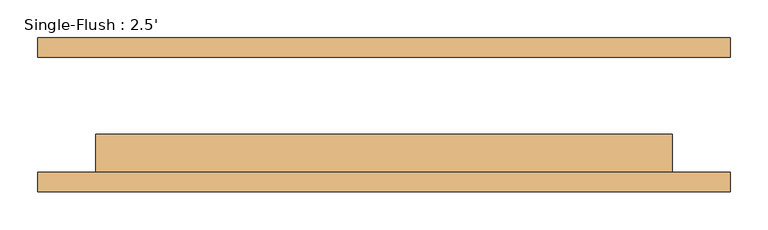
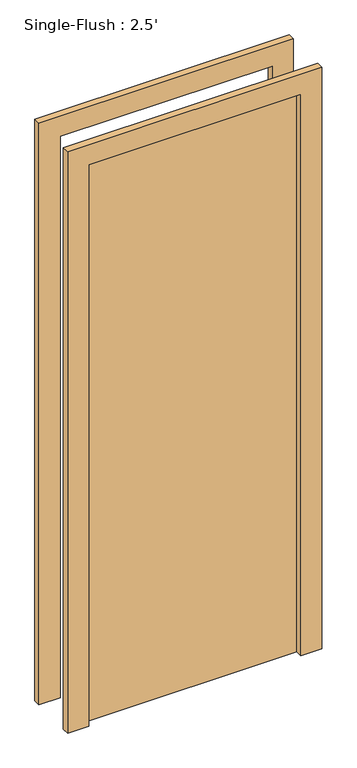
"""IFC4 building model written with IfcOpenShell, lengths in millimetres: door geometry, Single-Flush : 2.5'."""

from ifc_helpers import new_model, si_unit, frame, origin, origin_with_axes, place, context, project, spatial, polyline, outline, extrude, source, transform, mapped, element, save


def single_flush_2_5_e2b13fe9(model_context):
    return source(origin(), model_context, "Body", "SweptSolid", [
        extrude(outline(polyline([(2209.8, -457.2), (0.0, -457.2), (0.0, -381.0), (2133.6, -381.0), (2133.6, 381.0), (0.0, 381.0), (0.0, 457.2), (2209.8, 457.2), (2209.8, -457.2)])), frame((0.0, -101.6, 0.0), z_axis=(0.0, 1.0, 0.0), x_axis=(0.0, 0.0, 1.0)), (0.0, 0.0, 1.0), 25.4),
        extrude(outline(polyline([(2209.8, 457.2), (2209.8, -457.2), (0.0, -457.2), (0.0, -381.0), (2133.6, -381.0), (2133.6, 381.0), (0.0, 381.0), (0.0, 457.2), (2209.8, 457.2)])), frame((0.0, 76.2, 0.0), z_axis=(0.0, 1.0, 0.0), x_axis=(0.0, 0.0, 1.0)), (0.0, 0.0, 1.0), 25.4),
        extrude(outline(polyline([(381.0, -25.4), (381.0, -76.2), (-381.0, -76.2), (-381.0, -25.4), (381.0, -25.4)])), origin_with_axes(), (0.0, 0.0, 1.0), 2133.6),
    ])


if __name__ == "__main__":
    model = new_model("IFC4")
    model_context = context("Model", 3, world=origin())
    ifc_project = project(units=[si_unit("LENGTHUNIT", "METRE", prefix="MILLI")], contexts=[model_context])
    site = spatial("IfcSite", under=ifc_project)
    building = spatial("IfcBuilding", under=site)
    placement = place(None, origin())
    single_flush_2_5_shape = single_flush_2_5_e2b13fe9(model_context)
    element("IfcDoor", 1, ObjectType="Single-Flush : 2.5'", at=placement, inside=building, context=model_context, shape_type="MappedRepresentation", body=[
        mapped(single_flush_2_5_shape, transform((0.0, 0.0, 0.0), x_axis=(1.0, 0.0, 0.0), y_axis=(0.0, 1.0, 0.0), z_axis=(0.0, 0.0, 1.0))),
    ])
    save(model, "model.ifc")

# Revit data of these elements
# Type "Single-Flush : 2.5'"
#   Type Mark = "8"
#   Construction Type Id = "MDOOR"
#   Assembly Code = "C1020"
#   Analytic Construction = "Metal"
#   Thickness = 0' - 2"
#   Heat Transfer Coefficient (U) = 0.651978 BTU/(h·ft²·°F)
#   Height = 7' - 0"
#   Trim Projection Ext = 0' - 1"
#   Trim Projection Int = 0' - 1"
#   Trim Width = 0' - 3"
#   Width = 2' - 6"
#   Define Thermal Properties by = 1
#   Door Material = Door - Panel
#   Frame Material = Door - Frame
#   Visual Light Transmittance = 0
#   Solar Heat Gain Coefficient = 0
#   Function = (empty or 0)
#   Wall Closure = (empty or 0)
# Element 1 (IfcDoor, "Single-Flush : 2.5'")
#   Materials on its faces: "Door - Frame", "Door - Panel"
# Materials
#   "Door - Panel": class "Wood", colour RGB 210 159 95, transparency 0
#   "Door - Frame": colour RGB 118 70 51, transparency 0
